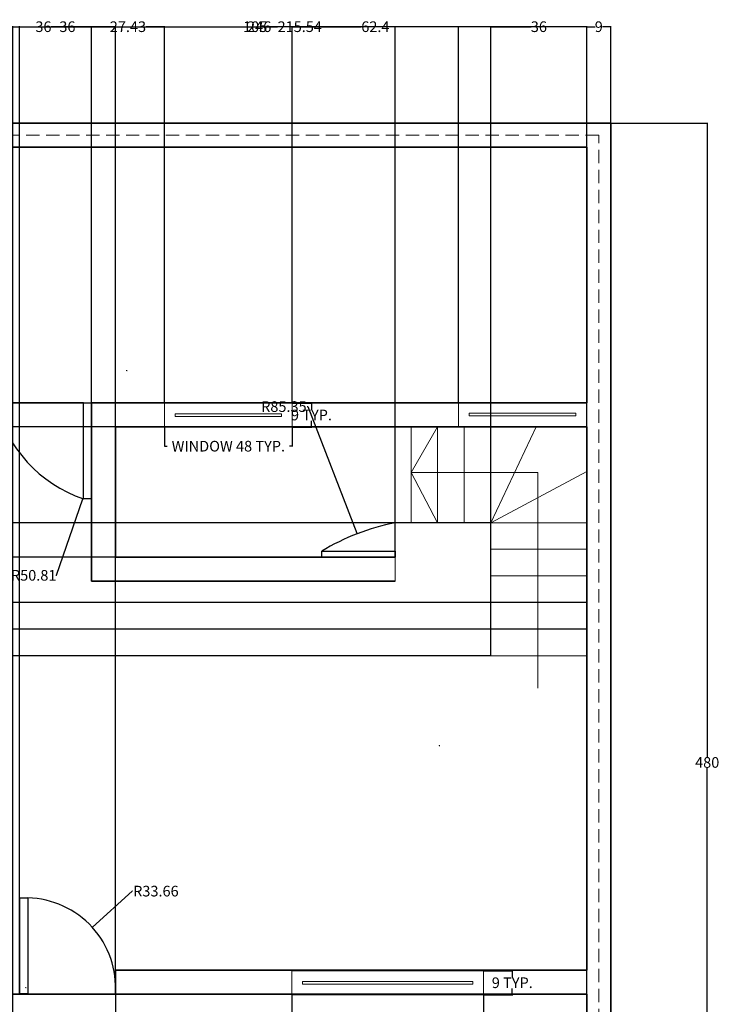
# Model space of a CAD drawing. Units: inches. Extents: x 1291 to 2095, y 532 to 1090.
# Tile 14 of 14: x 1832 to 2095, y 720 to 1090. Entities that reach past the tile are written whole.
import ezdxf

# ---------------------------------------------------------------- set-up
doc = ezdxf.new("R2010")
doc.units = ezdxf.units.IN
doc.header["$MEASUREMENT"] = 0
doc.linetypes.add('HIDDEN', pattern=[0.375, 0.25, -0.125])
for name, color, linetype, lineweight in [('A-ANNO-DIMS', 2, 'Continuous', 18), ('A-DOOR', 3, 'Continuous', 25), ('A-FLOR-STRS', 7, 'Continuous', 20), ('A-GLAZ', 4, 'Continuous', 18), ('A-WALL', 7, 'Continuous', 35), ('A-WALL-HIDN', 8, 'HIDDEN', 13)]:
    doc.layers.add(name, color=color, linetype=linetype, lineweight=lineweight)
doc.styles.get("Standard").update_dxf_attribs({"font": 'arial.ttf'})
doc.dimstyles.get("Standard").update_dxf_attribs({"dimtxt": 4, "dimasz": 0.18, "dimexe": 0.18, "dimexo": 0.0625, "dimgap": 0.09, "dimtad": 0, "dimtih": 1, "dimtoh": 1, "dimdec": 0, "dimrnd": 6, "dimzin": 0, "dimdsep": 46, "dimlunit": 3, "dimtxsty": 'Standard', "dimcen": 0.09, "dimadec": 0, "dimazin": 0, "dimtfac": 1, "dimtdec": 0, "dimtofl": 0, "dimtmove": 0, "dimatfit": 3, "dimfxl": 1, "dimtolj": 1, "dimtzin": 0, "dimarcsym": 0})

# ---------------------------------------------------------------- blocks, each defined once
blk = doc.blocks.new('WIN-72IN')
for points in [[(0, 0), (0, 9), (72, 9), (72, 0)], [(4, 4), (4, 5), (68, 5), (68, 4)]]:
    blk.add_lwpolyline(points, close=True)
blk = doc.blocks.new('WIN-48IN')
for points in [[(0, 0), (0, 9), (48, 9), (48, 0)], [(4, 4), (4, 5), (44, 5), (44, 4)]]:
    blk.add_lwpolyline(points, close=True)
blk = doc.blocks.new('*D12')
at = {"layer": 'A-ANNO-DIMS', "color": 0, "lineweight": -2, "transparency": 16777216}
for p, q in [((1934.29, 723.52), (1934.29, 712.6)), ((2006.29, 723.52), (2006.29, 712.6)), ((1934.47, 712.78), (1947.34, 712.78)), ((2006.11, 712.78), (1993.23, 712.78))]:
    blk.add_line(p, q, dxfattribs=at)
at = {"layer": 'A-ANNO-DIMS', "color": 0, "transparency": 16777216}
for points in [[(1934.47, 712.81), (1934.47, 712.75), (1934.29, 712.78)], [(2006.11, 712.81), (2006.11, 712.75), (2006.29, 712.78)]]:
    blk.add_solid(points, dxfattribs=at)
at = {"layer": 'Defpoints', "color": 0, "transparency": 16777216}
for p in [(1934.29, 723.58), (2006.29, 723.58), (2006.29, 712.78)]:
    blk.add_point(p, dxfattribs=at)
at = {"layer": 'A-ANNO-DIMS', "color": 0, "transparency": 16777216, "insert": (1970.29, 712.78), "char_height": 4, "attachment_point": 5}
blk.add_mtext('\\A1;WINDOW 72 TYP.', dxfattribs=at)
blk = doc.blocks.new('*D13')
at = {"layer": 'A-ANNO-DIMS', "color": 0, "lineweight": -2, "transparency": 16777216}
for p, q in [((2006.35, 732.58), (2017.27, 732.58)), ((2017.09, 732.4), (2017.09, 730.22)), ((2017.09, 723.76), (2017.09, 725.95)), ((2006.35, 723.58), (2017.27, 723.58))]:
    blk.add_line(p, q, dxfattribs=at)
at = {"layer": 'A-ANNO-DIMS', "color": 0, "transparency": 16777216}
for points in [[(2017.06, 732.4), (2017.12, 732.4), (2017.09, 732.58)], [(2017.06, 723.76), (2017.12, 723.76), (2017.09, 723.58)]]:
    blk.add_solid(points, dxfattribs=at)
at = {"layer": 'Defpoints', "color": 0, "transparency": 16777216}
for p in [(2006.29, 732.58), (2017.09, 732.58), (2006.29, 723.58)]:
    blk.add_point(p, dxfattribs=at)
at = {"layer": 'A-ANNO-DIMS', "color": 0, "transparency": 16777216, "insert": (2017.09, 728.08), "char_height": 4, "attachment_point": 5}
blk.add_mtext('\\A1;9 TYP.', dxfattribs=at)
blk = doc.blocks.new('*D14')
at = {"layer": 'A-ANNO-DIMS', "color": 0, "lineweight": -2, "transparency": 16777216}
for p, q in [((1886.5, 936.64), (1886.5, 929.32)), ((1934.5, 936.64), (1934.5, 929.32)), ((1886.68, 929.5), (1887.56, 929.5)), ((1934.32, 929.5), (1933.45, 929.5))]:
    blk.add_line(p, q, dxfattribs=at)
at = {"layer": 'A-ANNO-DIMS', "color": 0, "transparency": 16777216}
for points in [[(1886.68, 929.53), (1886.68, 929.47), (1886.5, 929.5)], [(1934.32, 929.53), (1934.32, 929.47), (1934.5, 929.5)]]:
    blk.add_solid(points, dxfattribs=at)
at = {"layer": 'Defpoints', "color": 0, "transparency": 16777216}
for p in [(1886.5, 936.7), (1934.5, 936.7), (1934.5, 929.5)]:
    blk.add_point(p, dxfattribs=at)
at = {"layer": 'A-ANNO-DIMS', "color": 0, "transparency": 16777216, "insert": (1910.5, 929.5), "char_height": 4, "attachment_point": 5}
blk.add_mtext('\\A1;WINDOW 48 TYP.', dxfattribs=at)
blk = doc.blocks.new('*D15')
at = {"layer": 'A-ANNO-DIMS', "color": 0, "lineweight": -2, "transparency": 16777216}
for p, q in [((1934.57, 945.7), (1941.88, 945.7)), ((1941.7, 945.52), (1941.7, 943.33)), ((1941.7, 936.88), (1941.7, 939.07)), ((1934.57, 936.7), (1941.88, 936.7))]:
    blk.add_line(p, q, dxfattribs=at)
at = {"layer": 'A-ANNO-DIMS', "color": 0, "transparency": 16777216}
for points in [[(1941.67, 945.52), (1941.73, 945.52), (1941.7, 945.7)], [(1941.67, 936.88), (1941.73, 936.88), (1941.7, 936.7)]]:
    blk.add_solid(points, dxfattribs=at)
at = {"layer": 'Defpoints', "color": 0, "transparency": 16777216}
for p in [(1934.5, 945.7), (1941.7, 945.7), (1934.5, 936.7)]:
    blk.add_point(p, dxfattribs=at)
at = {"layer": 'A-ANNO-DIMS', "color": 0, "transparency": 16777216, "insert": (1941.7, 941.2), "char_height": 4, "attachment_point": 5}
blk.add_mtext('\\A1;9 TYP.', dxfattribs=at)
blk = doc.blocks.new('*D33')
at = {"layer": 'A-ANNO-DIMS', "color": 0, "lineweight": -2, "transparency": 16777216}
for p, q in [((2054.14, 1050.78), (2090.45, 1050.78)), ((2090.27, 1050.6), (2090.27, 812.91)), ((2090.27, 570.96), (2090.27, 808.65)), ((2054.14, 570.78), (2090.45, 570.78))]:
    blk.add_line(p, q, dxfattribs=at)
at = {"layer": 'A-ANNO-DIMS', "color": 0, "transparency": 16777216}
for points in [[(2090.24, 1050.6), (2090.3, 1050.6), (2090.27, 1050.78)], [(2090.24, 570.96), (2090.3, 570.96), (2090.27, 570.78)]]:
    blk.add_solid(points, dxfattribs=at)
at = {"layer": 'Defpoints', "color": 0, "transparency": 16777216}
for p in [(2054.07, 1050.78), (2090.27, 1050.78), (2054.07, 570.78)]:
    blk.add_point(p, dxfattribs=at)
at = {"layer": 'A-ANNO-DIMS', "color": 0, "transparency": 16777216, "insert": (2090.27, 810.78), "char_height": 4, "attachment_point": 5}
blk.add_mtext('\\A1;480', dxfattribs=at)
blk = doc.blocks.new('*D42')
at = {"layer": 'A-ANNO-DIMS', "color": 0, "lineweight": -2, "transparency": 16777216}
for p, q in [((1799.07, 1041.84), (1799.07, 1087.16)), ((1799.25, 1086.98), (1917.53, 1086.98)), ((2044.89, 1086.98), (1926.62, 1086.98)), ((2045.07, 1041.84), (2045.07, 1087.16))]:
    blk.add_line(p, q, dxfattribs=at)
at = {"layer": 'A-ANNO-DIMS', "color": 0, "transparency": 16777216}
for points in [[(1799.25, 1087.01), (1799.25, 1086.95), (1799.07, 1086.98)], [(2044.89, 1087.01), (2044.89, 1086.95), (2045.07, 1086.98)]]:
    blk.add_solid(points, dxfattribs=at)
at = {"layer": 'Defpoints', "color": 0, "transparency": 16777216}
for p in [(2045.07, 1086.98), (1799.07, 1041.78), (2045.07, 1041.78)]:
    blk.add_point(p, dxfattribs=at)
at = {"layer": 'A-ANNO-DIMS', "color": 0, "transparency": 16777216, "insert": (1922.07, 1086.98), "char_height": 4, "attachment_point": 5}
blk.add_mtext('\\A1;246', dxfattribs=at)
blk = doc.blocks.new('*D43')
at = {"layer": 'A-ANNO-DIMS', "color": 0, "lineweight": -2, "transparency": 16777216}
for p, q in [((2045.07, 1041.84), (2045.07, 1087.16)), ((2045.25, 1086.98), (2048.17, 1086.98)), ((2053.89, 1086.98), (2050.98, 1086.98)), ((2054.07, 1050.84), (2054.07, 1087.16))]:
    blk.add_line(p, q, dxfattribs=at)
at = {"layer": 'A-ANNO-DIMS', "color": 0, "transparency": 16777216}
for points in [[(2045.25, 1087.01), (2045.25, 1086.95), (2045.07, 1086.98)], [(2053.89, 1087.01), (2053.89, 1086.95), (2054.07, 1086.98)]]:
    blk.add_solid(points, dxfattribs=at)
at = {"layer": 'Defpoints', "color": 0, "transparency": 16777216}
for p in [(2054.07, 1086.98), (2054.07, 1050.78), (2045.07, 1041.78)]:
    blk.add_point(p, dxfattribs=at)
at = {"layer": 'A-ANNO-DIMS', "color": 0, "transparency": 16777216, "insert": (2049.57, 1086.98), "char_height": 4, "attachment_point": 5}
blk.add_mtext('\\A1;9', dxfattribs=at)
blk = doc.blocks.new('*D45')
at = {"layer": 'A-ANNO-DIMS', "color": 0, "lineweight": -2, "transparency": 16777216}
for p, q in [((1829.54, 579.84), (1829.54, 1087.16)), ((1829.72, 1086.98), (1928.89, 1086.98)), ((2044.89, 1086.98), (1945.72, 1086.98)), ((2045.07, 579.84), (2045.07, 1087.16))]:
    blk.add_line(p, q, dxfattribs=at)
at = {"layer": 'A-ANNO-DIMS', "color": 0, "transparency": 16777216}
for points in [[(1829.72, 1087.01), (1829.72, 1086.95), (1829.54, 1086.98)], [(2044.89, 1087.01), (2044.89, 1086.95), (2045.07, 1086.98)]]:
    blk.add_solid(points, dxfattribs=at)
at = {"layer": 'Defpoints', "color": 0, "transparency": 16777216}
for p in [(2045.07, 1086.98), (1829.54, 579.78), (2045.07, 579.78)]:
    blk.add_point(p, dxfattribs=at)
at = {"layer": 'A-ANNO-DIMS', "color": 0, "transparency": 16777216, "insert": (1937.3, 1086.98), "char_height": 4, "attachment_point": 5}
blk.add_mtext('\\A1;215.54', dxfattribs=at)
blk = doc.blocks.new('*D55')
at = {"layer": 'A-ANNO-DIMS', "color": 0, "lineweight": -2, "transparency": 16777216}
for p, q in [((1868.07, 887.84), (1868.07, 1087.16)), ((1868.25, 1086.98), (1916.24, 1086.98)), ((1972.89, 1086.98), (1924.91, 1086.98)), ((1973.07, 887.84), (1973.07, 1087.16))]:
    blk.add_line(p, q, dxfattribs=at)
at = {"layer": 'A-ANNO-DIMS', "color": 0, "transparency": 16777216}
for points in [[(1868.25, 1087.01), (1868.25, 1086.95), (1868.07, 1086.98)], [(1972.89, 1087.01), (1972.89, 1086.95), (1973.07, 1086.98)]]:
    blk.add_solid(points, dxfattribs=at)
at = {"layer": 'Defpoints', "color": 0, "transparency": 16777216}
for p in [(1973.07, 1086.98), (1868.07, 887.78), (1973.07, 887.78)]:
    blk.add_point(p, dxfattribs=at)
at = {"layer": 'A-ANNO-DIMS', "color": 0, "transparency": 16777216, "insert": (1920.57, 1086.98), "char_height": 4, "attachment_point": 5}
blk.add_mtext('\\A1;105', dxfattribs=at)
blk = doc.blocks.new('*D56')
at = {"layer": 'A-ANNO-DIMS', "color": 0, "lineweight": -2, "transparency": 16777216}
for p, q in [((1868.01, 936.78), (1297.69, 936.78)), ((1297.87, 936.6), (1297.87, 914.41)), ((1297.87, 887.96), (1297.87, 910.15)), ((1868.01, 887.78), (1297.69, 887.78))]:
    blk.add_line(p, q, dxfattribs=at)
at = {"layer": 'A-ANNO-DIMS', "color": 0, "transparency": 16777216}
for points in [[(1297.84, 936.6), (1297.9, 936.6), (1297.87, 936.78)], [(1297.84, 887.96), (1297.9, 887.96), (1297.87, 887.78)]]:
    blk.add_solid(points, dxfattribs=at)
at = {"layer": 'Defpoints', "color": 0, "transparency": 16777216}
for p in [(1297.87, 936.78), (1868.07, 936.78), (1868.07, 887.78)]:
    blk.add_point(p, dxfattribs=at)
at = {"layer": 'A-ANNO-DIMS', "color": 0, "transparency": 16777216, "insert": (1297.87, 912.28), "char_height": 4, "attachment_point": 5}
blk.add_mtext('\\A1;49', dxfattribs=at)
blk = doc.blocks.new('*D57')
at = {"layer": 'A-ANNO-DIMS', "color": 0, "lineweight": -2, "transparency": 16777216}
for p, q in [((1973.01, 900.78), (1297.69, 900.78)), ((1297.87, 900.6), (1297.87, 896.41)), ((1297.87, 887.96), (1297.87, 892.15)), ((1973.01, 887.78), (1297.69, 887.78))]:
    blk.add_line(p, q, dxfattribs=at)
at = {"layer": 'A-ANNO-DIMS', "color": 0, "transparency": 16777216}
for points in [[(1297.84, 900.6), (1297.9, 900.6), (1297.87, 900.78)], [(1297.84, 887.96), (1297.9, 887.96), (1297.87, 887.78)]]:
    blk.add_solid(points, dxfattribs=at)
at = {"layer": 'Defpoints', "color": 0, "transparency": 16777216}
for p in [(1297.87, 900.78), (1973.07, 900.78), (1973.07, 887.78)]:
    blk.add_point(p, dxfattribs=at)
at = {"layer": 'A-ANNO-DIMS', "color": 0, "transparency": 16777216, "insert": (1297.87, 894.28), "char_height": 4, "attachment_point": 5}
blk.add_mtext('\\A1;13', dxfattribs=at)
blk = doc.blocks.new('*D58')
at = {"layer": 'A-ANNO-DIMS', "color": 0, "lineweight": -2, "transparency": 16777216}
for p, q in [((2009.07, 850.84), (2009.07, 1087.16)), ((2009.25, 1086.98), (2024.12, 1086.98)), ((2044.89, 1086.98), (2030.03, 1086.98)), ((2045.07, 850.84), (2045.07, 1087.16))]:
    blk.add_line(p, q, dxfattribs=at)
at = {"layer": 'A-ANNO-DIMS', "color": 0, "transparency": 16777216}
for points in [[(2009.25, 1087.01), (2009.25, 1086.95), (2009.07, 1086.98)], [(2044.89, 1087.01), (2044.89, 1086.95), (2045.07, 1086.98)]]:
    blk.add_solid(points, dxfattribs=at)
at = {"layer": 'Defpoints', "color": 0, "transparency": 16777216}
for p in [(2045.07, 1086.98), (2009.07, 850.78), (2045.07, 850.78)]:
    blk.add_point(p, dxfattribs=at)
at = {"layer": 'A-ANNO-DIMS', "color": 0, "transparency": 16777216, "insert": (2027.07, 1086.98), "char_height": 4, "attachment_point": 5}
blk.add_mtext('\\A1;36', dxfattribs=at)
blk = doc.blocks.new('*D59')
at = {"layer": 'A-ANNO-DIMS', "color": 0, "lineweight": -2, "transparency": 16777216}
for p, q in [((2009.01, 900.78), (1297.69, 900.78)), ((1297.87, 900.6), (1297.87, 877.91)), ((1297.87, 850.96), (1297.87, 873.65)), ((2009.01, 850.78), (1297.69, 850.78))]:
    blk.add_line(p, q, dxfattribs=at)
at = {"layer": 'A-ANNO-DIMS', "color": 0, "transparency": 16777216}
for points in [[(1297.84, 900.6), (1297.9, 900.6), (1297.87, 900.78)], [(1297.84, 850.96), (1297.9, 850.96), (1297.87, 850.78)]]:
    blk.add_solid(points, dxfattribs=at)
at = {"layer": 'Defpoints', "color": 0, "transparency": 16777216}
for p in [(1297.87, 900.78), (2009.07, 900.78), (2009.07, 850.78)]:
    blk.add_point(p, dxfattribs=at)
at = {"layer": 'A-ANNO-DIMS', "color": 0, "transparency": 16777216, "insert": (1297.87, 875.78), "char_height": 4, "attachment_point": 5}
blk.add_mtext('\\A1;50', dxfattribs=at)
blk = doc.blocks.new('*D60')
at = {"layer": 'A-ANNO-DIMS', "color": 0, "lineweight": -2, "transparency": 16777216}
for p, q in [((2045.01, 870.78), (1297.69, 870.78)), ((1297.87, 870.6), (1297.87, 867.91)), ((1297.87, 860.96), (1297.87, 863.65)), ((2045.01, 860.78), (1297.69, 860.78))]:
    blk.add_line(p, q, dxfattribs=at)
at = {"layer": 'A-ANNO-DIMS', "color": 0, "transparency": 16777216}
for points in [[(1297.84, 870.6), (1297.9, 870.6), (1297.87, 870.78)], [(1297.84, 860.96), (1297.9, 860.96), (1297.87, 860.78)]]:
    blk.add_solid(points, dxfattribs=at)
at = {"layer": 'Defpoints', "color": 0, "transparency": 16777216}
for p in [(1297.87, 870.78), (2045.07, 870.78), (2045.07, 860.78)]:
    blk.add_point(p, dxfattribs=at)
at = {"layer": 'A-ANNO-DIMS', "color": 0, "transparency": 16777216, "insert": (1297.87, 865.78), "char_height": 4, "attachment_point": 5}
blk.add_mtext('\\A1;10', dxfattribs=at)
blk = doc.blocks.new('*D67')
at = {"layer": 'A-ANNO-DIMS', "color": 0, "lineweight": -2, "transparency": 16777216}
for p, q in [((1832.07, 723.84), (1832.07, 1087.16)), ((1832.25, 1086.98), (1847.12, 1086.98)), ((1867.89, 1086.98), (1853.03, 1086.98)), ((1868.07, 723.84), (1868.07, 1087.16))]:
    blk.add_line(p, q, dxfattribs=at)
at = {"layer": 'A-ANNO-DIMS', "color": 0, "transparency": 16777216}
for points in [[(1832.25, 1087.01), (1832.25, 1086.95), (1832.07, 1086.98)], [(1867.89, 1087.01), (1867.89, 1086.95), (1868.07, 1086.98)]]:
    blk.add_solid(points, dxfattribs=at)
at = {"layer": 'Defpoints', "color": 0, "transparency": 16777216}
for p in [(1868.07, 1086.98), (1832.07, 723.78), (1868.07, 723.78)]:
    blk.add_point(p, dxfattribs=at)
at = {"layer": 'A-ANNO-DIMS', "color": 0, "transparency": 16777216, "insert": (1850.07, 1086.98), "char_height": 4, "attachment_point": 5}
blk.add_mtext('\\A1;36', dxfattribs=at)
blk = doc.blocks.new('*D68')
at = {"layer": 'A-ANNO-DIMS', "color": 0, "lineweight": -2, "transparency": 16777216}
for p, q in [((1868.07, 723.72), (1868.07, 534.4)), ((1934.29, 723.52), (1934.29, 534.4)), ((1868.25, 534.58), (1894.72, 534.58)), ((1934.11, 534.58), (1907.64, 534.58))]:
    blk.add_line(p, q, dxfattribs=at)
at = {"layer": 'A-ANNO-DIMS', "color": 0, "transparency": 16777216}
for points in [[(1868.25, 534.61), (1868.25, 534.55), (1868.07, 534.58)], [(1934.11, 534.61), (1934.11, 534.55), (1934.29, 534.58)]]:
    blk.add_solid(points, dxfattribs=at)
at = {"layer": 'Defpoints', "color": 0, "transparency": 16777216}
for p in [(1868.07, 723.78), (1934.29, 723.58), (1934.29, 534.58)]:
    blk.add_point(p, dxfattribs=at)
at = {"layer": 'A-ANNO-DIMS', "color": 0, "transparency": 16777216, "insert": (1901.18, 534.58), "char_height": 4, "attachment_point": 5}
blk.add_mtext('\\A1;66.21', dxfattribs=at)
blk = doc.blocks.new('*D75')
at = {"layer": 'A-ANNO-DIMS', "color": 0, "lineweight": -2, "transparency": 16777216}
for p, q in [((1823.07, 945.84), (1823.07, 1087.16)), ((1823.25, 1086.98), (1838.12, 1086.98)), ((1858.89, 1086.98), (1844.03, 1086.98)), ((1859.07, 945.84), (1859.07, 1087.16))]:
    blk.add_line(p, q, dxfattribs=at)
at = {"layer": 'A-ANNO-DIMS', "color": 0, "transparency": 16777216}
for points in [[(1823.25, 1087.01), (1823.25, 1086.95), (1823.07, 1086.98)], [(1858.89, 1087.01), (1858.89, 1086.95), (1859.07, 1086.98)]]:
    blk.add_solid(points, dxfattribs=at)
at = {"layer": 'Defpoints', "color": 0, "transparency": 16777216}
for p in [(1859.07, 1086.98), (1823.07, 945.78), (1859.07, 945.78)]:
    blk.add_point(p, dxfattribs=at)
at = {"layer": 'A-ANNO-DIMS', "color": 0, "transparency": 16777216, "insert": (1841.07, 1086.98), "char_height": 4, "attachment_point": 5}
blk.add_mtext('\\A1;36', dxfattribs=at)
blk = doc.blocks.new('*D76')
at = {"layer": 'A-ANNO-DIMS', "color": 0, "lineweight": -2, "transparency": 16777216}
for p, q in [((1859.07, 945.84), (1859.07, 1087.16)), ((1859.25, 1086.98), (1865.92, 1086.98)), ((1886.32, 1086.98), (1879.66, 1086.98)), ((1886.5, 945.76), (1886.5, 1087.16))]:
    blk.add_line(p, q, dxfattribs=at)
at = {"layer": 'A-ANNO-DIMS', "color": 0, "transparency": 16777216}
for points in [[(1859.25, 1087.01), (1859.25, 1086.95), (1859.07, 1086.98)], [(1886.32, 1087.01), (1886.32, 1086.95), (1886.5, 1086.98)]]:
    blk.add_solid(points, dxfattribs=at)
at = {"layer": 'Defpoints', "color": 0, "transparency": 16777216}
for p in [(1886.5, 1086.98), (1859.07, 945.78), (1886.5, 945.7)]:
    blk.add_point(p, dxfattribs=at)
at = {"layer": 'A-ANNO-DIMS', "color": 0, "transparency": 16777216, "insert": (1872.79, 1086.98), "char_height": 4, "attachment_point": 5}
blk.add_mtext('\\A1;27.43', dxfattribs=at)
blk = doc.blocks.new('*D77')
at = {"layer": 'A-ANNO-DIMS', "color": 0, "lineweight": -2, "transparency": 16777216}
for p, q in [((1934.5, 945.76), (1934.5, 1087.16)), ((1934.68, 1086.98), (1960.42, 1086.98)), ((1996.72, 1086.98), (1970.99, 1086.98)), ((1996.9, 945.9), (1996.9, 1087.16))]:
    blk.add_line(p, q, dxfattribs=at)
at = {"layer": 'A-ANNO-DIMS', "color": 0, "transparency": 16777216}
for points in [[(1934.68, 1087.01), (1934.68, 1086.95), (1934.5, 1086.98)], [(1996.72, 1087.01), (1996.72, 1086.95), (1996.9, 1086.98)]]:
    blk.add_solid(points, dxfattribs=at)
at = {"layer": 'Defpoints', "color": 0, "transparency": 16777216}
for p in [(1996.9, 1086.98), (1934.5, 945.7), (1996.9, 945.84)]:
    blk.add_point(p, dxfattribs=at)
at = {"layer": 'A-ANNO-DIMS', "color": 0, "transparency": 16777216, "insert": (1965.7, 1086.98), "char_height": 4, "attachment_point": 5}
blk.add_mtext('\\A1;62.4', dxfattribs=at)
blk = doc.blocks.new('*D84')
at = {"layer": 'A-ANNO-DIMS', "color": 0, "lineweight": -2, "transparency": 16777216}
for p, q in [((1940.1, 944.36), (1940.28, 944.36)), ((1940.28, 944.36), (1958.77, 896.8)), ((1989.67, 817.08), (1989.85, 817.08)), ((1989.76, 816.99), (1989.76, 817.17))]:
    blk.add_line(p, q, dxfattribs=at)
at = {"layer": 'A-ANNO-DIMS', "color": 0, "transparency": 16777216}
blk.add_solid([(1958.8, 896.81), (1958.75, 896.79), (1958.84, 896.63)], dxfattribs=at)
at = {"layer": 'Defpoints', "color": 0, "transparency": 16777216}
for p in [(1958.84, 896.63), (1989.76, 817.08)]:
    blk.add_point(p, dxfattribs=at)
at = {"layer": 'A-ANNO-DIMS', "color": 0, "transparency": 16777216, "insert": (1931.34, 944.36), "char_height": 4, "attachment_point": 5}
blk.add_mtext('\\A1;R85.35', dxfattribs=at)
blk = doc.blocks.new('*D87')
at = {"layer": 'A-ANNO-DIMS', "color": 0, "lineweight": -2, "transparency": 16777216}
for p, q in [((1874.36, 762.47), (1859.54, 749)), ((1874.54, 762.47), (1874.36, 762.47)), ((1834.41, 726.24), (1834.59, 726.24)), ((1834.5, 726.15), (1834.5, 726.33))]:
    blk.add_line(p, q, dxfattribs=at)
at = {"layer": 'A-ANNO-DIMS', "color": 0, "transparency": 16777216}
blk.add_solid([(1859.52, 749.03), (1859.56, 748.98), (1859.41, 748.88)], dxfattribs=at)
at = {"layer": 'Defpoints', "color": 0, "transparency": 16777216}
for p in [(1859.41, 748.88), (1834.5, 726.24)]:
    blk.add_point(p, dxfattribs=at)
at = {"layer": 'A-ANNO-DIMS', "color": 0, "transparency": 16777216, "insert": (1883.29, 762.47), "char_height": 4, "attachment_point": 5}
blk.add_mtext('\\A1;R33.66', dxfattribs=at)
blk = doc.blocks.new('*D91')
at = {"layer": 'A-ANNO-DIMS', "color": 0, "lineweight": -2, "transparency": 16777216}
for p, q in [((1872.33, 957.89), (1872.51, 957.89)), ((1872.42, 957.8), (1872.42, 957.98)), ((1845.96, 881.02), (1855.82, 909.68)), ((1845.78, 881.02), (1845.96, 881.02))]:
    blk.add_line(p, q, dxfattribs=at)
at = {"layer": 'A-ANNO-DIMS', "color": 0, "transparency": 16777216}
blk.add_solid([(1855.79, 909.69), (1855.85, 909.67), (1855.88, 909.85)], dxfattribs=at)
at = {"layer": 'Defpoints', "color": 0, "transparency": 16777216}
for p in [(1872.42, 957.89), (1855.88, 909.85)]:
    blk.add_point(p, dxfattribs=at)
at = {"layer": 'A-ANNO-DIMS', "color": 0, "transparency": 16777216, "insert": (1837.41, 881.02), "char_height": 4, "attachment_point": 5}
blk.add_mtext('\\A1;R50.81', dxfattribs=at)

msp = doc.modelspace()

# ---------------------------------------------------------------- linework, layer by layer
at = {"layer": 'A-DOOR'}
for points in [[(1856.0735, 945.7804), (1859.0735, 945.7804), (1859.0735, 909.7804), (1856.0735, 909.7804)], [(1973.0735, 890.0751), (1973.0735, 887.7804), (1945.5375, 887.7804), (1945.5375, 890.0751)], [(1832.2456, 759.8954), (1835.2456, 759.8954), (1835.2456, 723.8954), (1832.2456, 723.8954)]]:
    msp.add_lwpolyline(points, close=True, dxfattribs=at)
for centre, radius, start, end in [((1872.4221, 957.8916), 50.813, 193.789075, 251.231819), ((1989.7643, 817.082), 85.3464, 101.277748, 121.211886), ((1834.5006, 726.2407), 33.6629, 355.808674, 88.731965)]:
    msp.add_arc(centre, radius, start, end, dxfattribs=at)
at = {"layer": 'A-FLOR-STRS'}
for p, q in [((1973.0735, 878.7804), (1973.0735, 936.7804)), ((1979.0735, 900.7804), (1979.0735, 936.7804)), ((1979.0735, 919.6041), (1989.0735, 936.7804)), ((1989.0735, 900.7804), (1989.0735, 936.7804)), ((1999.0735, 900.7804), (1999.0735, 936.7804)), ((2009.0735, 850.7804), (2009.0735, 936.7804)), ((2009.0735, 900.7804), (2026.0123, 936.7804)), ((2026.7461, 919.6041), (1979.0735, 919.6041)), ((1979.0735, 919.6041), (1989.0735, 900.7804)), ((2009.0735, 900.7804), (2045.0735, 919.9494)), ((2026.7461, 838.706), (2026.7461, 919.6041)), ((2045.0735, 900.7804), (1973.0735, 900.7804)), ((2045.0735, 890.7804), (2009.0735, 890.7804)), ((2045.0735, 880.7804), (2009.0735, 880.7804)), ((2045.0735, 870.7804), (2009.0735, 870.7804)), ((2045.0735, 860.7804), (2009.0735, 860.7804)), ((2045.0735, 850.7804), (2009.0735, 850.7804))]:
    msp.add_line(p, q, dxfattribs=at)
at = {"layer": 'A-WALL'}
for p, q in [((2054.0735, 1050.7804), (1334.0735, 1050.7804)), ((2054.0735, 570.7804), (2054.0735, 1050.7804)), ((2045.0735, 1041.7804), (1703.0735, 1041.7804)), ((2045.0735, 945.7804), (2045.0735, 1041.7804)), ((1856.0735, 945.7804), (1703.0735, 945.7804)), ((2045.0735, 945.7804), (1859.0735, 945.7804)), ((1859.0735, 878.7804), (1859.0735, 945.7804)), ((2045.0735, 936.7804), (1868.0735, 936.7804)), ((1868.0735, 887.7804), (1868.0735, 936.7804)), ((2045.0735, 732.7804), (2045.0735, 936.7804)), ((1973.0735, 887.7804), (1868.0735, 887.7804)), ((1973.0735, 878.7804), (1859.0735, 878.7804)), ((1868.0735, 723.7804), (1868.0735, 732.7804)), ((1868.0735, 732.7804), (2045.0735, 732.7804)), ((1703.0735, 723.7804), (1868.0735, 723.7804)), ((1868.0735, 723.7804), (2045.0735, 723.7804)), ((2045.0735, 579.7804), (2045.0735, 723.7804))]:
    msp.add_line(p, q, dxfattribs=at)
at = {"layer": 'A-WALL-HIDN', "ltscale": 20}
for p, q in [((2049.5735, 1046.2804), (1338.5735, 1046.2804)), ((2049.5735, 570.7804), (2049.5735, 1046.2804))]:
    msp.add_line(p, q, dxfattribs=at)

# ---------------------------------------------------------------- block references
at = {"layer": 'A-GLAZ'}
for name, p in [('WIN-48IN', (1886.5042, 936.6989)), ('WIN-48IN', (1996.902, 936.836)), ('WIN-72IN', (1934.286, 723.585))]:
    msp.add_blockref(name, p, dxfattribs=at)

# ---------------------------------------------------------------- dimensions: what is measured, and where the dimension line sits
at = {"layer": 'A-ANNO-DIMS'}
for base, p1, p2, override, picture, middle in [((2045.0735, 1086.9804), (1799.0735, 1041.7804), (2045.0735, 1041.7804), {"dimdec": 0, "dimlfac": 1, "dimrnd": 0, "dimzin": 0, "dimdsep": 46, "dimlunit": 2}, '*D42', (1922.0735, 1086.9804)), ((1859.0735, 1086.9804), (1823.0735, 945.7804), (1859.0735, 945.7804), {"dimdec": 0, "dimlfac": 1, "dimrnd": 0, "dimzin": 0, "dimdsep": 46, "dimlunit": 2}, '*D75', (1841.0735, 1086.9804)), ((2045.0735, 1086.9804), (1829.5364, 579.7804), (2045.0735, 579.7804), {"dimdec": 2, "dimlfac": 1, "dimrnd": 0, "dimzin": 0, "dimdsep": 46, "dimlunit": 2}, '*D45', (1937.3049, 1086.9804)), ((1868.0735, 1086.9804), (1832.0735, 723.7804), (1868.0735, 723.7804), {"dimdec": 0, "dimlfac": 1, "dimrnd": 0, "dimzin": 0, "dimdsep": 46, "dimlunit": 2}, '*D67', (1850.0735, 1086.9804)), ((1886.5047, 1086.9804), (1859.0735, 945.7804), (1886.5047, 945.6993), {"dimdec": 2, "dimlfac": 1, "dimrnd": 0, "dimzin": 0, "dimdsep": 46, "dimlunit": 2}, '*D76', (1872.7891, 1086.9804)), ((1973.0735, 1086.9804), (1868.0735, 887.7804), (1973.0735, 887.7804), {"dimdec": 0, "dimlfac": 1, "dimrnd": 0, "dimzin": 0, "dimdsep": 46, "dimlunit": 2}, '*D55', (1920.5735, 1086.9804)), ((1996.9024, 1086.9804), (1934.5047, 945.6993), (1996.9024, 945.8364), {"dimdec": 1, "dimlfac": 1, "dimrnd": 0, "dimzin": 0, "dimdsep": 46, "dimlunit": 2}, '*D77', (1965.7035, 1086.9804)), ((2045.0735, 1086.9804), (2009.0735, 850.7804), (2045.0735, 850.7804), {"dimdec": 0, "dimlfac": 1, "dimrnd": 0, "dimzin": 0, "dimdsep": 46, "dimlunit": 2}, '*D58', (2027.0735, 1086.9804)), ((2054.0735, 1086.9804), (2045.0735, 1041.7804), (2054.0735, 1050.7804), {"dimdec": 0, "dimlfac": 1, "dimrnd": 0, "dimzin": 0, "dimdsep": 46, "dimlunit": 2}, '*D43', (2049.5735, 1086.9804)), ((1934.2856, 534.5804), (1868.0735, 723.7804), (1934.2856, 723.5846), {"dimdec": 2, "dimlfac": 1, "dimrnd": 0, "dimzin": 0, "dimdsep": 46, "dimlunit": 2}, '*D68', (1901.1796, 534.5804))]:
    dim = msp.add_linear_dim(base=base, p1=p1, p2=p2, dimstyle='Standard', override=override, dxfattribs=at)
    dim.commit()
    dim.dimension.update_dxf_attribs({"geometry": picture, "text_midpoint": middle})
for base, p1, p2, picture, middle in [((2090.2735, 1050.7804), (2054.0735, 570.7804), (2054.0735, 1050.7804), '*D33', (2090.2735, 810.7804)), ((1297.8735, 936.7804), (1868.0735, 887.7804), (1868.0735, 936.7804), '*D56', (1297.8735, 912.2804)), ((1297.8735, 900.7804), (1973.0735, 887.7804), (1973.0735, 900.7804), '*D57', (1297.8735, 894.2804)), ((1297.8735, 900.7804), (2009.0735, 850.7804), (2009.0735, 900.7804), '*D59', (1297.8735, 875.7804)), ((1297.8735, 870.7804), (2045.0735, 860.7804), (2045.0735, 870.7804), '*D60', (1297.8735, 865.7804))]:
    dim = msp.add_linear_dim(base=base, p1=p1, p2=p2, angle=90, dimstyle='Standard', override={"dimdec": 0, "dimlfac": 1, "dimrnd": 0, "dimzin": 0, "dimdsep": 46, "dimlunit": 2}, dxfattribs=at)
    dim.commit()
    dim.dimension.update_dxf_attribs({"geometry": picture, "text_midpoint": middle})
for center, mpoint, picture, middle in [((1872.4221, 957.8916), (1855.8814, 909.8461), '*D91', (1837.4101, 881.0188)), ((1989.7643, 817.082), (1958.8389, 896.6283), '*D84', (1931.3356, 944.3561)), ((1834.5006, 726.2407), (1859.4109, 748.8829), '*D87', (1883.2888, 762.4683))]:
    dim = msp.add_radius_dim(center=center, mpoint=mpoint, dimstyle='Standard', override={"dimdec": 2, "dimlfac": 1, "dimrnd": 0, "dimzin": 0, "dimdsep": 46, "dimlunit": 2}, dxfattribs=at)
    dim.commit()
    dim.dimension.update_dxf_attribs({"geometry": picture, "text_midpoint": middle, "dimtype": 164})
for base, p1, p2, picture, middle in [((1941.7047, 945.6993), (1934.5047, 936.6993), (1934.5047, 945.6993), '*D15', (1941.7047, 941.1993)), ((2017.0856, 732.5846), (2006.2856, 723.5846), (2006.2856, 732.5846), '*D13', (2017.0856, 728.0846))]:
    dim = msp.add_linear_dim(base=base, p1=p1, p2=p2, angle=90, text='<> TYP.', dimstyle='Standard', override={"dimdec": 0, "dimlfac": 1, "dimrnd": 0, "dimzin": 0, "dimdsep": 46, "dimlunit": 2}, dxfattribs=at)
    dim.commit()
    dim.dimension.update_dxf_attribs({"geometry": picture, "text_midpoint": middle})
for base, p1, p2, picture, middle in [((1934.5047, 929.4993), (1886.5047, 936.6993), (1934.5047, 936.6993), '*D14', (1910.5047, 929.4993)), ((2006.2856, 712.7846), (1934.2856, 723.5846), (2006.2856, 723.5846), '*D12', (1970.2856, 712.7846))]:
    dim = msp.add_linear_dim(base=base, p1=p1, p2=p2, text='WINDOW <> TYP.', dimstyle='Standard', override={"dimdec": 0, "dimlfac": 1, "dimrnd": 0, "dimzin": 0, "dimdsep": 46, "dimlunit": 2}, dxfattribs=at)
    dim.commit()
    dim.dimension.update_dxf_attribs({"geometry": picture, "text_midpoint": middle})

doc.saveas('drawing.dxf')
